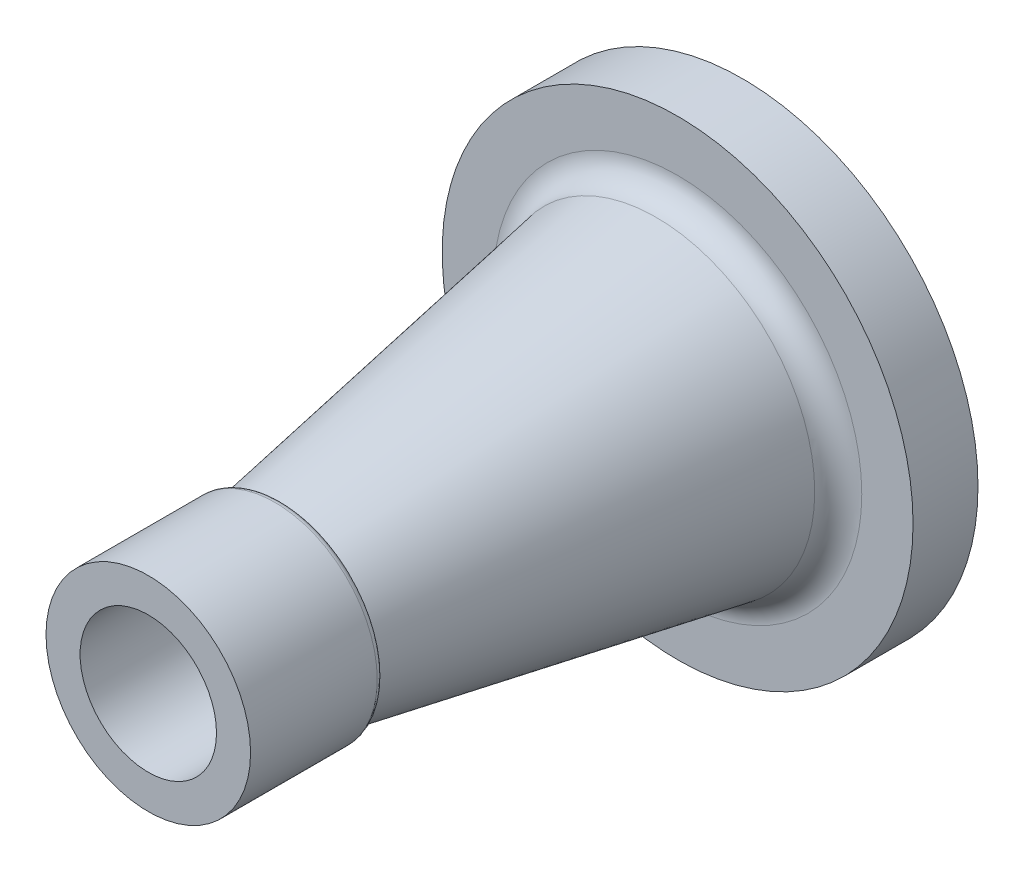
ISO-10303-21;
HEADER;
FILE_DESCRIPTION(('STEP AP214'),'2;1');
FILE_NAME('part.step','',(''),(''),'','','');
FILE_SCHEMA(('AUTOMOTIVE_DESIGN { 1 0 10303 214 1 1 1 1 }'));
ENDSEC;
DATA;
#1=APPLICATION_CONTEXT('core data for automotive mechanical design processes');
#2=APPLICATION_PROTOCOL_DEFINITION('international standard','automotive_design',2000,#1);
#3=PRODUCT_CONTEXT('',#1,'mechanical');
#4=PRODUCT('Part','Part','',(#3));
#5=PRODUCT_RELATED_PRODUCT_CATEGORY('part','',(#4));
#6=PRODUCT_DEFINITION_FORMATION('','',#4);
#7=PRODUCT_DEFINITION_CONTEXT('part definition',#1,'design');
#8=PRODUCT_DEFINITION('design','',#6,#7);
#9=PRODUCT_DEFINITION_SHAPE('','',#8);
#10=(LENGTH_UNIT() NAMED_UNIT(*) SI_UNIT(.MILLI.,.METRE.));
#11=(NAMED_UNIT(*) PLANE_ANGLE_UNIT() SI_UNIT($,.RADIAN.));
#12=(NAMED_UNIT(*) SI_UNIT($,.STERADIAN.) SOLID_ANGLE_UNIT());
#13=UNCERTAINTY_MEASURE_WITH_UNIT(LENGTH_MEASURE(1.E-05),#10,'distance_accuracy_value','');
#14=(GEOMETRIC_REPRESENTATION_CONTEXT(3) GLOBAL_UNCERTAINTY_ASSIGNED_CONTEXT((#13)) GLOBAL_UNIT_ASSIGNED_CONTEXT((#10,
#11,#12)) REPRESENTATION_CONTEXT('',''));
#15=CARTESIAN_POINT('',(0.,0.,0.));
#16=DIRECTION('',(0.,0.,1.));
#17=DIRECTION('',(1.,0.,0.));
#18=AXIS2_PLACEMENT_3D('',#15,#16,#17);
#19=CARTESIAN_POINT('',(0.,0.,20.));
#20=DIRECTION('',(0.,0.,-1.));
#21=DIRECTION('',(1.,0.,0.));
#22=AXIS2_PLACEMENT_3D('',#19,#20,#21);
#23=CONICAL_SURFACE('',#22,50.,0.174532925199433);
#24=CARTESIAN_POINT('',(0.,0.,26.6108145786645));
#25=DIRECTION('',(0.,0.,1.));
#26=DIRECTION('',(1.,0.,0.));
#27=AXIS2_PLACEMENT_3D('',#24,#25,#26);
#28=CIRCLE('',#27,48.8343350253206);
#29=CARTESIAN_POINT('',(48.8343350253206,0.,26.6108145786645));
#30=VERTEX_POINT('',#29);
#31=EDGE_CURVE('E55',#30,#30,#28,.T.);
#32=ORIENTED_EDGE('',*,*,#31,.T.);
#33=EDGE_LOOP('',(#32));
#34=FACE_BOUND('',#33,.T.);
#35=CARTESIAN_POINT('',(0.,0.,142.));
#36=DIRECTION('',(0.,0.,1.));
#37=DIRECTION('',(1.,0.,0.));
#38=AXIS2_PLACEMENT_3D('',#35,#36,#37);
#39=CIRCLE('',#38,28.4881083535673);
#40=CARTESIAN_POINT('',(28.4881083535673,0.,142.));
#41=VERTEX_POINT('',#40);
#42=EDGE_CURVE('E60',#41,#41,#39,.T.);
#43=ORIENTED_EDGE('',*,*,#42,.F.);
#44=EDGE_LOOP('',(#43));
#45=FACE_BOUND('',#44,.T.);
#46=ADVANCED_FACE('F40',(#34,#45),#23,.T.);
#47=CARTESIAN_POINT('',(0.,0.,20.));
#48=DIRECTION('',(0.,0.,-1.));
#49=DIRECTION('',(-1.,0.,0.));
#50=AXIS2_PLACEMENT_3D('',#47,#48,#49);
#51=CYLINDRICAL_SURFACE('',#50,72.5);
#52=CARTESIAN_POINT('',(0.,0.,20.));
#53=DIRECTION('',(0.,0.,1.));
#54=DIRECTION('',(1.,0.,0.));
#55=AXIS2_PLACEMENT_3D('',#52,#53,#54);
#56=CIRCLE('',#55,72.5);
#57=CARTESIAN_POINT('',(72.5,0.,20.));
#58=VERTEX_POINT('',#57);
#59=EDGE_CURVE('E58',#58,#58,#56,.T.);
#60=ORIENTED_EDGE('',*,*,#59,.F.);
#61=EDGE_LOOP('',(#60));
#62=FACE_BOUND('',#61,.T.);
#63=CARTESIAN_POINT('',(0.,0.,0.));
#64=DIRECTION('',(0.,0.,1.));
#65=DIRECTION('',(1.,0.,0.));
#66=AXIS2_PLACEMENT_3D('',#63,#64,#65);
#67=CIRCLE('',#66,72.5);
#68=CARTESIAN_POINT('',(72.5,0.,0.));
#69=VERTEX_POINT('',#68);
#70=EDGE_CURVE('E61',#69,#69,#67,.T.);
#71=ORIENTED_EDGE('',*,*,#70,.T.);
#72=EDGE_LOOP('',(#71));
#73=FACE_BOUND('',#72,.T.);
#74=ADVANCED_FACE('F106',(#62,#73),#51,.T.);
#75=CARTESIAN_POINT('',(0.,0.,20.));
#76=DIRECTION('',(0.,0.,1.));
#77=DIRECTION('',(1.,0.,0.));
#78=AXIS2_PLACEMENT_3D('',#75,#76,#77);
#79=PLANE('',#78);
#80=CARTESIAN_POINT('',(0.,0.,20.));
#81=DIRECTION('',(0.,0.,1.));
#82=DIRECTION('',(1.,0.,0.));
#83=AXIS2_PLACEMENT_3D('',#80,#81,#82);
#84=CIRCLE('',#83,56.7127970494182);
#85=CARTESIAN_POINT('',(56.7127970494182,0.,20.));
#86=VERTEX_POINT('',#85);
#87=EDGE_CURVE('E48',#86,#86,#84,.F.);
#88=ORIENTED_EDGE('',*,*,#87,.T.);
#89=EDGE_LOOP('',(#88));
#90=FACE_BOUND('',#89,.T.);
#91=ORIENTED_EDGE('',*,*,#59,.T.);
#92=EDGE_LOOP('',(#91));
#93=FACE_BOUND('',#92,.T.);
#94=ADVANCED_FACE('F101',(#90,#93),#79,.T.);
#95=CARTESIAN_POINT('',(0.,0.,0.));
#96=DIRECTION('',(0.,0.,1.));
#97=DIRECTION('',(1.,0.,0.));
#98=AXIS2_PLACEMENT_3D('',#95,#96,#97);
#99=PLANE('',#98);
#100=ORIENTED_EDGE('',*,*,#70,.F.);
#101=EDGE_LOOP('',(#100));
#102=FACE_BOUND('',#101,.T.);
#103=ADVANCED_FACE('F91',(#102),#99,.F.);
#104=CARTESIAN_POINT('',(0.,0.,142.));
#105=DIRECTION('',(0.,0.,1.));
#106=DIRECTION('',(1.,0.,0.));
#107=AXIS2_PLACEMENT_3D('',#104,#105,#106);
#108=CYLINDRICAL_SURFACE('',#107,31.5);
#109=CARTESIAN_POINT('',(0.,0.,144.));
#110=DIRECTION('',(0.,0.,1.));
#111=DIRECTION('',(1.,0.,0.));
#112=AXIS2_PLACEMENT_3D('',#109,#110,#111);
#113=CIRCLE('',#112,31.5);
#114=CARTESIAN_POINT('',(31.5,0.,144.));
#115=VERTEX_POINT('',#114);
#116=EDGE_CURVE('E42',#115,#115,#113,.T.);
#117=ORIENTED_EDGE('',*,*,#116,.T.);
#118=EDGE_LOOP('',(#117));
#119=FACE_BOUND('',#118,.T.);
#120=CARTESIAN_POINT('',(0.,0.,183.));
#121=DIRECTION('',(0.,0.,1.));
#122=DIRECTION('',(1.,0.,0.));
#123=AXIS2_PLACEMENT_3D('',#120,#121,#122);
#124=CIRCLE('',#123,31.5);
#125=CARTESIAN_POINT('',(31.5,0.,183.));
#126=VERTEX_POINT('',#125);
#127=EDGE_CURVE('E63',#126,#126,#124,.T.);
#128=ORIENTED_EDGE('',*,*,#127,.F.);
#129=EDGE_LOOP('',(#128));
#130=FACE_BOUND('',#129,.T.);
#131=ADVANCED_FACE('F93',(#119,#130),#108,.T.);
#132=CARTESIAN_POINT('',(0.,0.,142.));
#133=DIRECTION('',(0.,0.,1.));
#134=DIRECTION('',(1.,0.,0.));
#135=AXIS2_PLACEMENT_3D('',#132,#133,#134);
#136=PLANE('',#135);
#137=CARTESIAN_POINT('',(0.,0.,142.));
#138=DIRECTION('',(0.,0.,1.));
#139=DIRECTION('',(1.,0.,0.));
#140=AXIS2_PLACEMENT_3D('',#137,#138,#139);
#141=CIRCLE('',#140,29.5);
#142=CARTESIAN_POINT('',(29.5,0.,142.));
#143=VERTEX_POINT('',#142);
#144=EDGE_CURVE('E10',#143,#143,#141,.F.);
#145=ORIENTED_EDGE('',*,*,#144,.T.);
#146=EDGE_LOOP('',(#145));
#147=FACE_BOUND('',#146,.T.);
#148=ORIENTED_EDGE('',*,*,#42,.T.);
#149=EDGE_LOOP('',(#148));
#150=FACE_BOUND('',#149,.T.);
#151=ADVANCED_FACE('F87',(#147,#150),#136,.F.);
#152=CARTESIAN_POINT('',(0.,0.,183.));
#153=DIRECTION('',(0.,0.,1.));
#154=DIRECTION('',(1.,0.,0.));
#155=AXIS2_PLACEMENT_3D('',#152,#153,#154);
#156=PLANE('',#155);
#157=CARTESIAN_POINT('',(0.,0.,183.));
#158=DIRECTION('',(0.,0.,1.));
#159=DIRECTION('',(1.,0.,0.));
#160=AXIS2_PLACEMENT_3D('',#157,#158,#159);
#161=CIRCLE('',#160,21.);
#162=CARTESIAN_POINT('',(21.,0.,183.));
#163=VERTEX_POINT('',#162);
#164=EDGE_CURVE('E68',#163,#163,#161,.T.);
#165=ORIENTED_EDGE('',*,*,#164,.F.);
#166=EDGE_LOOP('',(#165));
#167=FACE_BOUND('',#166,.T.);
#168=ORIENTED_EDGE('',*,*,#127,.T.);
#169=EDGE_LOOP('',(#168));
#170=FACE_BOUND('',#169,.T.);
#171=ADVANCED_FACE('F82',(#167,#170),#156,.T.);
#172=CARTESIAN_POINT('',(0.,0.,25.));
#173=DIRECTION('',(0.,0.,1.));
#174=DIRECTION('',(1.,0.,0.));
#175=AXIS2_PLACEMENT_3D('',#172,#173,#174);
#176=CYLINDRICAL_SURFACE('',#175,21.);
#177=CARTESIAN_POINT('',(0.,0.,25.));
#178=DIRECTION('',(0.,0.,1.));
#179=DIRECTION('',(1.,0.,0.));
#180=AXIS2_PLACEMENT_3D('',#177,#178,#179);
#181=CIRCLE('',#180,21.);
#182=CARTESIAN_POINT('',(21.,0.,25.));
#183=VERTEX_POINT('',#182);
#184=EDGE_CURVE('E66',#183,#183,#181,.T.);
#185=ORIENTED_EDGE('',*,*,#184,.F.);
#186=EDGE_LOOP('',(#185));
#187=FACE_BOUND('',#186,.T.);
#188=ORIENTED_EDGE('',*,*,#164,.T.);
#189=EDGE_LOOP('',(#188));
#190=FACE_BOUND('',#189,.T.);
#191=ADVANCED_FACE('F79',(#187,#190),#176,.F.);
#192=CARTESIAN_POINT('',(0.,0.,25.));
#193=DIRECTION('',(0.,0.,1.));
#194=DIRECTION('',(1.,0.,0.));
#195=AXIS2_PLACEMENT_3D('',#192,#193,#194);
#196=PLANE('',#195);
#197=ORIENTED_EDGE('',*,*,#184,.T.);
#198=EDGE_LOOP('',(#197));
#199=FACE_BOUND('',#198,.T.);
#200=ADVANCED_FACE('F76',(#199),#196,.T.);
#201=CARTESIAN_POINT('',(0.,0.,28.));
#202=DIRECTION('',(0.,0.,1.));
#203=DIRECTION('',(1.,0.,0.));
#204=AXIS2_PLACEMENT_3D('',#201,#202,#203);
#205=TOROIDAL_SURFACE('',#204,56.7127970494182,8.);
#206=ORIENTED_EDGE('',*,*,#87,.F.);
#207=EDGE_LOOP('',(#206));
#208=FACE_BOUND('',#207,.T.);
#209=ORIENTED_EDGE('',*,*,#31,.F.);
#210=EDGE_LOOP('',(#209));
#211=FACE_BOUND('',#210,.T.);
#212=ADVANCED_FACE('F119',(#208,#211),#205,.F.);
#213=CARTESIAN_POINT('',(0.,0.,144.));
#214=DIRECTION('',(0.,0.,1.));
#215=DIRECTION('',(1.,0.,0.));
#216=AXIS2_PLACEMENT_3D('',#213,#214,#215);
#217=TOROIDAL_SURFACE('',#216,29.5,2.);
#218=ORIENTED_EDGE('',*,*,#144,.F.);
#219=EDGE_LOOP('',(#218));
#220=FACE_BOUND('',#219,.T.);
#221=ORIENTED_EDGE('',*,*,#116,.F.);
#222=EDGE_LOOP('',(#221));
#223=FACE_BOUND('',#222,.T.);
#224=ADVANCED_FACE('F39',(#220,#223),#217,.T.);
#225=CLOSED_SHELL('',(#46,#74,#94,#103,#131,#151,#171,#191,#200,#212,#224));
#226=MANIFOLD_SOLID_BREP('B2',#225);
#227=ADVANCED_BREP_SHAPE_REPRESENTATION('',(#18,#226),#14);
#228=SHAPE_DEFINITION_REPRESENTATION(#9,#227);
ENDSEC;
END-ISO-10303-21;
